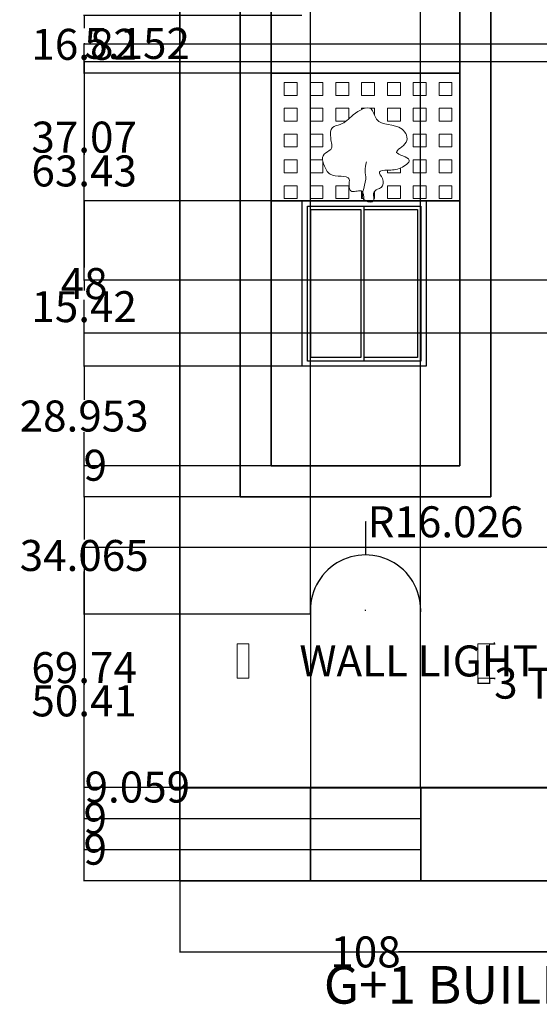
# Model space of a CAD drawing. Units: inches. Extents: x -30 to 323, y -174 to 256.
# Tile 1 of 4: x -24 to 127, y -174 to 112. Entities that reach past the tile are written whole.
import ezdxf

# ---------------------------------------------------------------- set-up
doc = ezdxf.new("R2010")
doc.units = ezdxf.units.IN
doc.header["$MEASUREMENT"] = 0
for name, color, linetype, lineweight in [('A-ANNO-DIMS', 2, 'Continuous', 18), ('A-ANNO-TEXT', 7, 'Continuous', 25), ('A-DOOR', 4, 'Continuous', 25), ('A-ELEV', 7, 'Continuous', 35), ('A-ELEV-PATT', 8, 'Continuous', 13), ('A-FLOR-STRS', 7, 'Continuous', 25), ('A-GLAZ', 3, 'Continuous', 25), ('E-LITE', 6, 'Continuous', 18), ('L-PLNT', 3, 'Continuous', 18)]:
    doc.layers.add(name, color=color, linetype=linetype, lineweight=lineweight)
doc.styles.get("Standard").update_dxf_attribs({"font": 'arial.ttf'})
doc.dimstyles.get("Standard").update_dxf_attribs({"dimtxt": 9, "dimasz": 0.18, "dimexe": 0.18, "dimexo": 0.0625, "dimgap": 0.09, "dimtad": 0, "dimtih": 1, "dimtoh": 1, "dimdec": 0, "dimzin": 0, "dimdsep": 46, "dimlunit": 3, "dimtxsty": 'Standard', "dimcen": 0.09, "dimadec": 0, "dimazin": 0, "dimtfac": 1, "dimtdec": 0, "dimtofl": 0, "dimtmove": 0, "dimatfit": 3, "dimfxl": 1, "dimtolj": 1, "dimtzin": 0, "dimarcsym": 0})

# ---------------------------------------------------------------- blocks, each defined once
blk = doc.blocks.new('*U2')
for p, q in [((1.5, 1.5), (1.5, 46.5)), ((1.5, 46.5), (18, 46.5)), ((18, 1.5), (18, 46.5)), ((18, 46.5), (34.5, 46.5)), ((34.5, 46.5), (34.5, 1.5)), ((18, 1.5), (1.5, 1.5)), ((34.5, 1.5), (18, 1.5))]:
    blk.add_line(p, q)
blk.add_lwpolyline([(0, 0), (0, 48), (36, 48), (36, 0)], close=True)
for points in [[(17, 45.5), (17, 2.5), (2.5, 2.5), (2.5, 45.5), (17, 45.5)], [(18, 45.5), (33.5, 45.5), (33.5, 2.5), (18, 2.5)]]:
    blk.add_lwpolyline(points)
blk = doc.blocks.new('WALL-LIGHT')
blk.add_lwpolyline([(0, 9.92), (3.36, 9.92), (3.36, 0), (0, 0)], close=True)
blk = doc.blocks.new('*D7')
at = {"layer": 'A-ANNO-DIMS', "color": 0, "lineweight": -2, "transparency": 16777216}
for p, q in [((112.24, -69.33), (113.85, -69.33)), ((113.67, -69.15), (113.67, -68.97)), ((112.24, -79.25), (113.85, -79.25)), ((113.67, -79.43), (113.67, -79.61))]:
    blk.add_line(p, q, dxfattribs=at)
at = {"layer": 'A-ANNO-DIMS', "color": 0, "transparency": 16777216}
for points in [[(113.64, -69.15), (113.7, -69.15), (113.67, -69.33)], [(113.64, -79.43), (113.7, -79.43), (113.67, -79.25)]]:
    blk.add_solid(points, dxfattribs=at)
at = {"layer": 'Defpoints', "color": 0, "transparency": 16777216}
for p in [(112.18, -69.33), (113.67, -69.33), (112.18, -79.25)]:
    blk.add_point(p, dxfattribs=at)
at = {"layer": 'A-ANNO-DIMS', "color": 0, "transparency": 16777216, "insert": (113.67, -74.29), "char_height": 9, "attachment_point": 5}
blk.add_mtext('\\A1;WALL LIGHT 10 TYP.', dxfattribs=at)
blk = doc.blocks.new('*D8')
at = {"layer": 'A-ANNO-DIMS', "color": 0, "lineweight": -2, "transparency": 16777216}
for p, q in [((108.82, -79.31), (108.82, -80.91)), ((112.18, -79.31), (112.18, -80.91)), ((109, -80.73), (112, -80.73)), ((112.18, -80.73), (112.36, -80.73))]:
    blk.add_line(p, q, dxfattribs=at)
at = {"layer": 'A-ANNO-DIMS', "color": 0, "transparency": 16777216}
for points in [[(109, -80.7), (109, -80.76), (108.82, -80.73)], [(112, -80.7), (112, -80.76), (112.18, -80.73)]]:
    blk.add_solid(points, dxfattribs=at)
at = {"layer": 'Defpoints', "color": 0, "transparency": 16777216}
for p in [(108.82, -79.25), (112.18, -79.25), (112.18, -80.73)]:
    blk.add_point(p, dxfattribs=at)
at = {"layer": 'A-ANNO-DIMS', "color": 0, "transparency": 16777216, "insert": (130.85, -80.73), "char_height": 9, "attachment_point": 5}
blk.add_mtext('\\A1;3 TYP.', dxfattribs=at)
blk = doc.blocks.new('*D9')
at = {"layer": 'A-ANNO-DIMS', "color": 0, "lineweight": -2, "transparency": 16777216}
for p, q in [((283.63, 8.84), (283.63, -158.98)), ((22.14, -138.22), (22.14, -158.98)), ((22.32, -158.8), (137.5, -158.8)), ((283.45, -158.8), (168.27, -158.8))]:
    blk.add_line(p, q, dxfattribs=at)
at = {"layer": 'A-ANNO-DIMS', "color": 0, "transparency": 16777216}
for points in [[(22.32, -158.77), (22.32, -158.83), (22.14, -158.8)], [(283.45, -158.77), (283.45, -158.83), (283.63, -158.8)]]:
    blk.add_solid(points, dxfattribs=at)
at = {"layer": 'Defpoints', "color": 0, "transparency": 16777216}
for p in [(283.63, 8.91), (22.14, -138.15), (283.63, -158.8)]:
    blk.add_point(p, dxfattribs=at)
at = {"layer": 'A-ANNO-DIMS', "color": 0, "transparency": 16777216, "insert": (152.88, -158.8), "char_height": 9, "attachment_point": 5}
blk.add_mtext('\\A1;261.5', dxfattribs=at)
blk = doc.blocks.new('*D10')
at = {"layer": 'A-ANNO-DIMS', "color": 0, "lineweight": -2, "transparency": 16777216}
for p, q in [((15.03, 229.9), (304.46, 229.9)), ((304.28, 229.72), (304.28, 50.56)), ((304.28, -137.97), (304.28, 41.18)), ((22.2, -138.15), (304.46, -138.15))]:
    blk.add_line(p, q, dxfattribs=at)
at = {"layer": 'A-ANNO-DIMS', "color": 0, "transparency": 16777216}
for points in [[(304.25, 229.72), (304.31, 229.72), (304.28, 229.9)], [(304.25, -137.97), (304.31, -137.97), (304.28, -138.15)]]:
    blk.add_solid(points, dxfattribs=at)
at = {"layer": 'Defpoints', "color": 0, "transparency": 16777216}
for p in [(14.97, 229.9), (22.14, -138.15), (304.28, -138.15)]:
    blk.add_point(p, dxfattribs=at)
at = {"layer": 'A-ANNO-DIMS', "color": 0, "transparency": 16777216, "insert": (304.28, 45.87), "char_height": 9, "attachment_point": 5}
blk.add_mtext('\\A1;368.05', dxfattribs=at)
blk = doc.blocks.new('*D21')
at = {"layer": 'A-ANNO-DIMS', "color": 0, "lineweight": -2, "transparency": 16777216}
for p, q in [((22.14, -111.03), (22.14, 250.73)), ((22.32, 250.55), (25.92, 250.55)), ((59.97, 250.55), (56.37, 250.55)), ((60.15, -60.62), (60.15, 250.73))]:
    blk.add_line(p, q, dxfattribs=at)
at = {"layer": 'A-ANNO-DIMS', "color": 0, "transparency": 16777216}
for points in [[(22.32, 250.58), (22.32, 250.52), (22.14, 250.55)], [(59.97, 250.58), (59.97, 250.52), (60.15, 250.55)]]:
    blk.add_solid(points, dxfattribs=at)
at = {"layer": 'Defpoints', "color": 0, "transparency": 16777216}
for p in [(60.15, 250.55), (60.15, -60.68), (22.14, -111.09)]:
    blk.add_point(p, dxfattribs=at)
at = {"layer": 'A-ANNO-DIMS', "color": 0, "transparency": 16777216, "insert": (41.14, 250.55), "char_height": 9, "attachment_point": 5}
blk.add_mtext('\\A1;38.02', dxfattribs=at)
blk = doc.blocks.new('*D22')
at = {"layer": 'A-ANNO-DIMS', "color": 0, "lineweight": -2, "transparency": 16777216}
for p, q in [((92.12, -60.62), (92.12, 250.73)), ((92.3, 250.55), (95.9, 250.55)), ((129.96, 250.55), (126.35, 250.55)), ((130.14, -111.03), (130.14, 250.73))]:
    blk.add_line(p, q, dxfattribs=at)
at = {"layer": 'A-ANNO-DIMS', "color": 0, "transparency": 16777216}
for points in [[(92.3, 250.58), (92.3, 250.52), (92.12, 250.55)], [(129.96, 250.58), (129.96, 250.52), (130.14, 250.55)]]:
    blk.add_solid(points, dxfattribs=at)
at = {"layer": 'Defpoints', "color": 0, "transparency": 16777216}
for p in [(130.14, 250.55), (92.12, -60.68), (130.14, -111.09)]:
    blk.add_point(p, dxfattribs=at)
at = {"layer": 'A-ANNO-DIMS', "color": 0, "transparency": 16777216, "insert": (111.13, 250.55), "char_height": 9, "attachment_point": 5}
blk.add_mtext('\\A1;38.02', dxfattribs=at)
blk = doc.blocks.new('*D23')
at = {"layer": 'A-ANNO-DIMS', "color": 0, "lineweight": -2, "transparency": 16777216}
for p, q in [((22.14, -138.22), (22.14, -158.98)), ((130.14, -138.22), (130.14, -158.98)), ((22.32, -158.8), (66.52, -158.8)), ((129.96, -158.8), (85.75, -158.8))]:
    blk.add_line(p, q, dxfattribs=at)
at = {"layer": 'A-ANNO-DIMS', "color": 0, "transparency": 16777216}
for points in [[(22.32, -158.77), (22.32, -158.83), (22.14, -158.8)], [(129.96, -158.77), (129.96, -158.83), (130.14, -158.8)]]:
    blk.add_solid(points, dxfattribs=at)
at = {"layer": 'Defpoints', "color": 0, "transparency": 16777216}
for p in [(22.14, -138.15), (130.14, -138.15), (130.14, -158.8)]:
    blk.add_point(p, dxfattribs=at)
at = {"layer": 'A-ANNO-DIMS', "color": 0, "transparency": 16777216, "insert": (76.14, -158.8), "char_height": 9, "attachment_point": 5}
blk.add_mtext('\\A1;108', dxfattribs=at)
blk = doc.blocks.new('*D24')
at = {"layer": 'A-ANNO-DIMS', "color": 0, "lineweight": -2, "transparency": 16777216}
for p, q in [((60.09, -129.15), (-5.86, -129.15)), ((-5.68, -129.15), (-5.68, -128.97)), ((-5.68, -128.97), (-5.5, -128.97)), ((-5.68, -137.97), (-5.68, -129.33)), ((22.07, -138.15), (-5.86, -138.15))]:
    blk.add_line(p, q, dxfattribs=at)
at = {"layer": 'A-ANNO-DIMS', "color": 0, "transparency": 16777216}
for points in [[(-5.71, -129.33), (-5.65, -129.33), (-5.68, -129.15)], [(-5.71, -137.97), (-5.65, -137.97), (-5.68, -138.15)]]:
    blk.add_solid(points, dxfattribs=at)
at = {"layer": 'Defpoints', "color": 0, "transparency": 16777216}
for p in [(-5.68, -129.15), (60.15, -129.15), (22.14, -138.15)]:
    blk.add_point(p, dxfattribs=at)
at = {"layer": 'A-ANNO-DIMS', "color": 0, "transparency": 16777216, "insert": (-2.45, -128.97), "char_height": 9, "attachment_point": 5}
blk.add_mtext('\\A1;9', dxfattribs=at)
blk = doc.blocks.new('*D25')
at = {"layer": 'A-ANNO-DIMS', "color": 0, "lineweight": -2, "transparency": 16777216}
for p, q in [((-5.68, -120.15), (-5.68, -119.97)), ((-5.68, -119.97), (-5.5, -119.97)), ((60.09, -120.15), (-5.86, -120.15)), ((-5.68, -128.97), (-5.68, -120.33)), ((60.09, -129.15), (-5.86, -129.15))]:
    blk.add_line(p, q, dxfattribs=at)
at = {"layer": 'A-ANNO-DIMS', "color": 0, "transparency": 16777216}
for points in [[(-5.71, -120.33), (-5.65, -120.33), (-5.68, -120.15)], [(-5.71, -128.97), (-5.65, -128.97), (-5.68, -129.15)]]:
    blk.add_solid(points, dxfattribs=at)
at = {"layer": 'Defpoints', "color": 0, "transparency": 16777216}
for p in [(-5.68, -120.15), (60.15, -120.15), (60.15, -129.15)]:
    blk.add_point(p, dxfattribs=at)
at = {"layer": 'A-ANNO-DIMS', "color": 0, "transparency": 16777216, "insert": (-2.45, -119.97), "char_height": 9, "attachment_point": 5}
blk.add_mtext('\\A1;9', dxfattribs=at)
blk = doc.blocks.new('*D26')
at = {"layer": 'A-ANNO-DIMS', "color": 0, "lineweight": -2, "transparency": 16777216}
for p, q in [((22.07, -111.09), (-5.86, -111.09)), ((-5.68, -111.09), (-5.68, -110.91)), ((-5.68, -110.91), (-5.5, -110.91)), ((-5.68, -119.97), (-5.68, -111.27)), ((60.09, -120.15), (-5.86, -120.15))]:
    blk.add_line(p, q, dxfattribs=at)
at = {"layer": 'A-ANNO-DIMS', "color": 0, "transparency": 16777216}
for points in [[(-5.71, -111.27), (-5.65, -111.27), (-5.68, -111.09)], [(-5.71, -119.97), (-5.65, -119.97), (-5.68, -120.15)]]:
    blk.add_solid(points, dxfattribs=at)
at = {"layer": 'Defpoints', "color": 0, "transparency": 16777216}
for p in [(-5.68, -111.09), (22.14, -111.09), (60.15, -120.15)]:
    blk.add_point(p, dxfattribs=at)
at = {"layer": 'A-ANNO-DIMS', "color": 0, "transparency": 16777216, "insert": (9.78, -110.91), "char_height": 9, "attachment_point": 5}
blk.add_mtext('\\A1;9.059', dxfattribs=at)
blk = doc.blocks.new('*D27')
at = {"layer": 'A-ANNO-DIMS', "color": 0, "lineweight": -2, "transparency": 16777216}
for p, q in [((60.09, -60.68), (-5.86, -60.68)), ((-5.68, -60.86), (-5.68, -81.2)), ((-5.68, -110.91), (-5.68, -90.57)), ((22.07, -111.09), (-5.86, -111.09))]:
    blk.add_line(p, q, dxfattribs=at)
at = {"layer": 'A-ANNO-DIMS', "color": 0, "transparency": 16777216}
for points in [[(-5.71, -60.86), (-5.65, -60.86), (-5.68, -60.68)], [(-5.71, -110.91), (-5.65, -110.91), (-5.68, -111.09)]]:
    blk.add_solid(points, dxfattribs=at)
at = {"layer": 'Defpoints', "color": 0, "transparency": 16777216}
for p in [(-5.68, -60.68), (60.15, -60.68), (22.14, -111.09)]:
    blk.add_point(p, dxfattribs=at)
at = {"layer": 'A-ANNO-DIMS', "color": 0, "transparency": 16777216, "insert": (-5.68, -85.89), "char_height": 9, "attachment_point": 5}
blk.add_mtext('\\A1;50.41', dxfattribs=at)
blk = doc.blocks.new('*D28')
at = {"layer": 'A-ANNO-DIMS', "color": 0, "lineweight": -2, "transparency": 16777216}
for p, q in [((39.63, -26.62), (-5.86, -26.62)), ((-5.68, -26.8), (-5.68, -38.96)), ((-5.68, -60.5), (-5.68, -48.34)), ((60.09, -60.68), (-5.86, -60.68))]:
    blk.add_line(p, q, dxfattribs=at)
at = {"layer": 'A-ANNO-DIMS', "color": 0, "transparency": 16777216}
for points in [[(-5.71, -26.8), (-5.65, -26.8), (-5.68, -26.62)], [(-5.71, -60.5), (-5.65, -60.5), (-5.68, -60.68)]]:
    blk.add_solid(points, dxfattribs=at)
at = {"layer": 'Defpoints', "color": 0, "transparency": 16777216}
for p in [(-5.68, -26.62), (39.69, -26.62), (60.15, -60.68)]:
    blk.add_point(p, dxfattribs=at)
at = {"layer": 'A-ANNO-DIMS', "color": 0, "transparency": 16777216, "insert": (-5.68, -43.65), "char_height": 9, "attachment_point": 5}
blk.add_mtext('\\A1;34.065', dxfattribs=at)
blk = doc.blocks.new('*D29')
at = {"layer": 'A-ANNO-DIMS', "color": 0, "lineweight": -2, "transparency": 16777216}
for p, q in [((48.63, -17.62), (-5.86, -17.62)), ((-5.68, -17.62), (-5.68, -17.44)), ((-5.68, -17.44), (-5.5, -17.44)), ((-5.68, -26.44), (-5.68, -17.8)), ((39.63, -26.62), (-5.86, -26.62))]:
    blk.add_line(p, q, dxfattribs=at)
at = {"layer": 'A-ANNO-DIMS', "color": 0, "transparency": 16777216}
for points in [[(-5.71, -17.8), (-5.65, -17.8), (-5.68, -17.62)], [(-5.71, -26.44), (-5.65, -26.44), (-5.68, -26.62)]]:
    blk.add_solid(points, dxfattribs=at)
at = {"layer": 'Defpoints', "color": 0, "transparency": 16777216}
for p in [(-5.68, -17.62), (48.69, -17.62), (39.69, -26.62)]:
    blk.add_point(p, dxfattribs=at)
at = {"layer": 'A-ANNO-DIMS', "color": 0, "transparency": 16777216, "insert": (-2.45, -17.44), "char_height": 9, "attachment_point": 5}
blk.add_mtext('\\A1;9', dxfattribs=at)
blk = doc.blocks.new('*D30')
at = {"layer": 'A-ANNO-DIMS', "color": 0, "lineweight": -2, "transparency": 16777216}
for p, q in [((57.66, 11.33), (-5.86, 11.33)), ((-5.68, 11.15), (-5.68, 1.55)), ((-5.68, -17.44), (-5.68, -7.83)), ((48.63, -17.62), (-5.86, -17.62))]:
    blk.add_line(p, q, dxfattribs=at)
at = {"layer": 'A-ANNO-DIMS', "color": 0, "transparency": 16777216}
for points in [[(-5.71, 11.15), (-5.65, 11.15), (-5.68, 11.33)], [(-5.71, -17.44), (-5.65, -17.44), (-5.68, -17.62)]]:
    blk.add_solid(points, dxfattribs=at)
at = {"layer": 'Defpoints', "color": 0, "transparency": 16777216}
for p in [(-5.68, 11.33), (57.72, 11.33), (48.69, -17.62)]:
    blk.add_point(p, dxfattribs=at)
at = {"layer": 'A-ANNO-DIMS', "color": 0, "transparency": 16777216, "insert": (-5.68, -3.14), "char_height": 9, "attachment_point": 5}
blk.add_mtext('\\A1;28.953', dxfattribs=at)
blk = doc.blocks.new('*D31')
at = {"layer": 'A-ANNO-DIMS', "color": 0, "lineweight": -2, "transparency": 16777216}
for p, q in [((48.63, 59.33), (-5.86, 59.33)), ((-5.68, 59.15), (-5.68, 40.02)), ((-5.68, 11.51), (-5.68, 30.65)), ((57.66, 11.33), (-5.86, 11.33))]:
    blk.add_line(p, q, dxfattribs=at)
at = {"layer": 'A-ANNO-DIMS', "color": 0, "transparency": 16777216}
for points in [[(-5.71, 59.15), (-5.65, 59.15), (-5.68, 59.33)], [(-5.71, 11.51), (-5.65, 11.51), (-5.68, 11.33)]]:
    blk.add_solid(points, dxfattribs=at)
at = {"layer": 'Defpoints', "color": 0, "transparency": 16777216}
for p in [(-5.68, 59.33), (48.7, 59.33), (57.72, 11.33)]:
    blk.add_point(p, dxfattribs=at)
at = {"layer": 'A-ANNO-DIMS', "color": 0, "transparency": 16777216, "insert": (-5.68, 35.33), "char_height": 9, "attachment_point": 5}
blk.add_mtext('\\A1;48', dxfattribs=at)
blk = doc.blocks.new('*D32')
at = {"layer": 'A-ANNO-DIMS', "color": 0, "lineweight": -2, "transparency": 16777216}
for p, q in [((48.63, 96.41), (-5.86, 96.41)), ((-5.68, 96.23), (-5.68, 82.56)), ((-5.68, 59.51), (-5.68, 73.18)), ((48.63, 59.33), (-5.86, 59.33))]:
    blk.add_line(p, q, dxfattribs=at)
at = {"layer": 'A-ANNO-DIMS', "color": 0, "transparency": 16777216}
for points in [[(-5.71, 96.23), (-5.65, 96.23), (-5.68, 96.41)], [(-5.71, 59.51), (-5.65, 59.51), (-5.68, 59.33)]]:
    blk.add_solid(points, dxfattribs=at)
at = {"layer": 'Defpoints', "color": 0, "transparency": 16777216}
for p in [(-5.68, 96.41), (48.7, 96.41), (48.7, 59.33)]:
    blk.add_point(p, dxfattribs=at)
at = {"layer": 'A-ANNO-DIMS', "color": 0, "transparency": 16777216, "insert": (-5.68, 77.87), "char_height": 9, "attachment_point": 5}
blk.add_mtext('\\A1;37.07', dxfattribs=at)
blk = doc.blocks.new('*D33')
at = {"layer": 'A-ANNO-DIMS', "color": 0, "lineweight": -2, "transparency": 16777216}
for p, q in [((57.66, 113.23), (-5.86, 113.23)), ((-5.68, 113.05), (-5.68, 109.5)), ((-5.68, 96.59), (-5.68, 100.13)), ((48.63, 96.41), (-5.86, 96.41))]:
    blk.add_line(p, q, dxfattribs=at)
at = {"layer": 'A-ANNO-DIMS', "color": 0, "transparency": 16777216}
for points in [[(-5.71, 113.05), (-5.65, 113.05), (-5.68, 113.23)], [(-5.71, 96.59), (-5.65, 96.59), (-5.68, 96.41)]]:
    blk.add_solid(points, dxfattribs=at)
at = {"layer": 'Defpoints', "color": 0, "transparency": 16777216}
for p in [(-5.68, 113.23), (57.72, 113.23), (48.7, 96.41)]:
    blk.add_point(p, dxfattribs=at)
at = {"layer": 'A-ANNO-DIMS', "color": 0, "transparency": 16777216, "insert": (-5.68, 104.82), "char_height": 9, "attachment_point": 5}
blk.add_mtext('\\A1;16.82', dxfattribs=at)
blk = doc.blocks.new('*D61')
at = {"layer": 'A-ANNO-DIMS', "color": 0, "lineweight": -2, "transparency": 16777216}
for p, q in [((148.07, -41.35), (-5.86, -41.35)), ((-5.68, -41.53), (-5.68, -71.54)), ((-5.68, -110.91), (-5.68, -80.91)), ((130.07, -111.09), (-5.86, -111.09))]:
    blk.add_line(p, q, dxfattribs=at)
at = {"layer": 'A-ANNO-DIMS', "color": 0, "transparency": 16777216}
for points in [[(-5.71, -41.53), (-5.65, -41.53), (-5.68, -41.35)], [(-5.71, -110.91), (-5.65, -110.91), (-5.68, -111.09)]]:
    blk.add_solid(points, dxfattribs=at)
at = {"layer": 'Defpoints', "color": 0, "transparency": 16777216}
for p in [(-5.68, -41.35), (148.14, -41.35), (130.14, -111.09)]:
    blk.add_point(p, dxfattribs=at)
at = {"layer": 'A-ANNO-DIMS', "color": 0, "transparency": 16777216, "insert": (-5.68, -76.22), "char_height": 9, "attachment_point": 5}
blk.add_mtext('\\A1;69.74', dxfattribs=at)
blk = doc.blocks.new('*D74')
at = {"layer": 'A-ANNO-DIMS', "color": 0, "lineweight": -2, "transparency": 16777216}
for p, q in [((145.92, 36.33), (-5.86, 36.33)), ((-5.68, 36.15), (-5.68, 33.3)), ((-5.68, 21.09), (-5.68, 23.93)), ((142.07, 20.91), (-5.86, 20.91))]:
    blk.add_line(p, q, dxfattribs=at)
at = {"layer": 'A-ANNO-DIMS', "color": 0, "transparency": 16777216}
for points in [[(-5.71, 36.15), (-5.65, 36.15), (-5.68, 36.33)], [(-5.71, 21.09), (-5.65, 21.09), (-5.68, 20.91)]]:
    blk.add_solid(points, dxfattribs=at)
at = {"layer": 'Defpoints', "color": 0, "transparency": 16777216}
for p in [(-5.68, 36.33), (145.99, 36.33), (142.14, 20.91)]:
    blk.add_point(p, dxfattribs=at)
at = {"layer": 'A-ANNO-DIMS', "color": 0, "transparency": 16777216, "insert": (-5.68, 28.62), "char_height": 9, "attachment_point": 5}
blk.add_mtext('\\A1;15.42', dxfattribs=at)
blk = doc.blocks.new('*D75')
at = {"layer": 'A-ANNO-DIMS', "color": 0, "lineweight": -2, "transparency": 16777216}
for p, q in [((145.92, 99.75), (-5.86, 99.75)), ((-5.68, 99.57), (-5.68, 72.73)), ((-5.68, 36.51), (-5.68, 63.35)), ((145.92, 36.33), (-5.86, 36.33))]:
    blk.add_line(p, q, dxfattribs=at)
at = {"layer": 'A-ANNO-DIMS', "color": 0, "transparency": 16777216}
for points in [[(-5.71, 99.57), (-5.65, 99.57), (-5.68, 99.75)], [(-5.71, 36.51), (-5.65, 36.51), (-5.68, 36.33)]]:
    blk.add_solid(points, dxfattribs=at)
at = {"layer": 'Defpoints', "color": 0, "transparency": 16777216}
for p in [(-5.68, 99.75), (145.99, 99.75), (145.99, 36.33)]:
    blk.add_point(p, dxfattribs=at)
at = {"layer": 'A-ANNO-DIMS', "color": 0, "transparency": 16777216, "insert": (-5.68, 68.04), "char_height": 9, "attachment_point": 5}
blk.add_mtext('\\A1;63.43', dxfattribs=at)
blk = doc.blocks.new('*D76')
at = {"layer": 'A-ANNO-DIMS', "color": 0, "lineweight": -2, "transparency": 16777216}
for p, q in [((142.07, 104.91), (-5.86, 104.91)), ((-5.68, 104.91), (-5.68, 105.09)), ((-5.68, 105.09), (-5.5, 105.09)), ((-5.68, 99.93), (-5.68, 104.73)), ((145.92, 99.75), (-5.86, 99.75))]:
    blk.add_line(p, q, dxfattribs=at)
at = {"layer": 'A-ANNO-DIMS', "color": 0, "transparency": 16777216}
for points in [[(-5.71, 104.73), (-5.65, 104.73), (-5.68, 104.91)], [(-5.71, 99.93), (-5.65, 99.93), (-5.68, 99.75)]]:
    blk.add_solid(points, dxfattribs=at)
at = {"layer": 'Defpoints', "color": 0, "transparency": 16777216}
for p in [(-5.68, 104.91), (142.14, 104.91), (145.99, 99.75)]:
    blk.add_point(p, dxfattribs=at)
at = {"layer": 'A-ANNO-DIMS', "color": 0, "transparency": 16777216, "insert": (9.73, 105.09), "char_height": 9, "attachment_point": 5}
blk.add_mtext('\\A1;5.152', dxfattribs=at)
blk = doc.blocks.new('*D77')
at = {"layer": 'A-ANNO-DIMS', "color": 0, "lineweight": -2, "transparency": 16777216}
for p, q in [((76.32, -33.87), (76.14, -33.87)), ((76.14, -33.87), (76.14, -43.3)), ((76.05, -59.51), (76.23, -59.51)), ((76.14, -59.6), (76.14, -59.42))]:
    blk.add_line(p, q, dxfattribs=at)
at = {"layer": 'A-ANNO-DIMS', "color": 0, "transparency": 16777216}
blk.add_solid([(76.11, -43.3), (76.17, -43.3), (76.14, -43.48)], dxfattribs=at)
at = {"layer": 'Defpoints', "color": 0, "transparency": 16777216}
for p in [(76.14, -43.48), (76.14, -59.51)]:
    blk.add_point(p, dxfattribs=at)
at = {"layer": 'A-ANNO-DIMS', "color": 0, "transparency": 16777216, "insert": (99.39, -33.87), "char_height": 9, "attachment_point": 5}
blk.add_mtext('\\A1;R16.026', dxfattribs=at)

msp = doc.modelspace()

# ---------------------------------------------------------------- hatches: boundary and pattern name
at = {"layer": 'A-ELEV-PATT'}
h = msp.add_hatch(dxfattribs=at)
h.set_pattern_fill('SQUARE', color=256, scale=30)
edge = h.paths.add_edge_path()
edge.add_spline(control_points=[(75.3211, 61.7995), (75.1986, 62.0071), (74.4578, 62.6896), (71.738, 61.3333), (71.2119, 63.9023), (72.0257, 67.3627), (66.4586, 65.797), (64.2082, 69.0428), (62.6837, 72.8814), (66.9111, 74.1759), (65.8088, 77.508), (65.831, 81.0228), (69.831, 81.5148), (72.1684, 84.4623), (78.0553, 87.8418), (79.2681, 80.5196), (86.2826, 82.5145), (89.4686, 76.0117), (82.5196, 73.1865), (90.9262, 71.7358), (85.7413, 68.2966), (83.5112, 68.3268), (79.2817, 68.145), (81.5493, 65.7412), (81.2688, 63.2947), (79.4617, 62.7519), (77.8918, 61.5997), (78.7703, 59.7999), (78.4437, 59.334)], knot_values=[2.20389569, 2.20389569, 2.20389569, 2.20389569, 3.0333133, 5.96980343, 7.60712091, 9.50541194, 15.20272299, 16.79439629, 21.50478909, 23.85346698, 27.13233668, 30.28156068, 32.68718212, 37.38454327, 42.8463849, 46.16655969, 54.15254193, 58.13701982, 62.16754012, 66.43266235, 69.73131729, 73.76374154, 76.06819784, 78.15373141, 80.76526319, 81.92378142, 83.63296344, 85.8374237, 85.8374237, 85.8374237, 85.8374237], degree=3, periodic=0)
edge.add_line((78.4437, 59.334), (93.7226, 59.334))
edge.add_line((93.7226, 59.334), (103.581, 59.334))
edge.add_line((103.581, 59.334), (103.5822, 96.4058))
edge.add_line((103.5822, 96.4058), (48.6979, 96.4058))
edge.add_line((48.6979, 96.4058), (48.6966, 59.334))
edge.add_line((48.6966, 59.334), (75.7226, 59.334))
edge.add_spline(control_points=[(75.7226, 59.334), (75.7185, 59.4366), (75.7144, 59.5392), (75.71, 59.6412)], knot_values=[0, 0, 0, 0, 0.23624815, 0.23624815, 0.23624815, 0.23624815], degree=3, periodic=0)
edge.add_spline(control_points=[(75.71, 59.6412), (75.1902, 60.1562), (75.1644, 60.926), (75.3211, 61.7995)], knot_values=[88.68438083, 88.68438083, 88.68438083, 88.68438083, 91.0965344, 91.0965344, 91.0965344, 91.0965344], degree=3, periodic=0)

# ---------------------------------------------------------------- linework, layer by layer
at = {"layer": 'A-DOOR'}
msp.add_lwpolyline([(60.1531, -60.6838), (60.1531, -111.0941), (92.1189, -111.0941), (92.1189, -60.6838, 1.07623618)], format="xyb", close=True, dxfattribs=at)
at = {"layer": 'A-ELEV'}
for p, q in [((39.6938, -26.6189), (39.7012, 195.2341)), ((112.5855, 195.2341), (112.5782, -26.6189)), ((48.6941, -17.6189), (48.7009, 186.2341)), ((103.5852, 186.2341), (103.5785, -17.6189)), ((103.5785, -17.6189), (48.6941, -17.6189)), ((112.5782, -26.6189), (39.6938, -26.6189))]:
    msp.add_line(p, q, dxfattribs=at)
msp.add_lwpolyline([(130.136, 149.9059), (274.136, 149.9059), (274.136, 128.9059), (279.5695, 128.9059), (279.5695, 104.9059), (274.136, 104.9059), (274.136, 20.9059), (283.6325, 20.9059), (283.6325, 8.9059), (274.136, 8.9059), (274.136, -111.0941), (22.136, -111.0941), (22.136, 224.9059), (130.136, 224.9059), (130.136, -111.0941)], dxfattribs=at)
for points in [[(48.6966, 59.334), (103.5822, 59.334), (103.5822, 96.4058), (48.6966, 96.4058)], [(60.1531, -111.0941), (22.136, -111.0941), (22.136, -138.1526), (60.1531, -138.1526)], [(92.2427, -111.0941), (130.136, -111.0941), (130.136, -138.1526), (92.2427, -138.1526)]]:
    msp.add_lwpolyline(points, close=True, dxfattribs=at)
at = {"layer": 'A-FLOR-STRS'}
for p, q in [((60.1531, -138.1526), (60.1531, -111.0941)), ((92.2427, -111.0941), (92.2427, -138.1526)), ((92.2427, -120.1526), (60.1531, -120.1526)), ((92.2427, -129.1526), (60.1531, -129.1526)), ((92.2427, -138.1526), (60.1531, -138.1526))]:
    msp.add_line(p, q, dxfattribs=at)
at = {"layer": 'L-PLNT'}
msp.add_open_spline([(75.7226, 59.334), (75.6702, 60.651), (75.5671, 63.2427), (71.738, 61.3333), (71.2119, 63.9023), (72.0257, 67.3627), (66.4586, 65.797), (64.2082, 69.0428), (62.6837, 72.8814), (66.9111, 74.1759), (65.8088, 77.508), (65.831, 81.0228), (69.831, 81.5148), (72.1684, 84.4623), (78.0553, 87.8418), (79.2681, 80.5196), (86.2826, 82.5145), (89.4686, 76.0117), (82.5196, 73.1865), (90.9262, 71.7358), (85.7413, 68.2966), (83.5112, 68.3268), (79.2817, 68.145), (81.5493, 65.7412), (81.2688, 63.2947), (79.4617, 62.7519), (77.8918, 61.5997), (79.2875, 58.7402), (73.4514, 59.2667), (76.786, 64.556), (75.8288, 68.1331), (76.1857, 69.8132), (76.3709, 70.6848)], degree=3, knots=[0, 0, 0, 0, 3.0333133, 5.96980343, 7.60712091, 9.50541194, 15.20272299, 16.79439629, 21.50478909, 23.85346698, 27.13233668, 30.28156068, 32.68718212, 37.38454327, 42.8463849, 46.16655969, 54.15254193, 58.13701982, 62.16754012, 66.43266235, 69.73131729, 73.76374154, 76.06819784, 78.15373141, 80.76526319, 81.92378142, 83.63296344, 85.8374237, 88.14168399, 94.48814382, 96.91031937, 99.52185115, 99.52185115, 99.52185115, 99.52185115], dxfattribs=at)

# ---------------------------------------------------------------- block references
at = {"layer": 'A-GLAZ'}
msp.add_blockref('*U2', (57.7226, 11.334), dxfattribs=at)
at = {"layer": 'E-LITE'}
for p in [(38.841, -79.246), (108.8156, -79.246)]:
    msp.add_blockref('WALL-LIGHT', p, dxfattribs=at)

# ---------------------------------------------------------------- texts
at = {"layer": 'A-ANNO-TEXT'}
msp.add_text('G+1 BUILDING ELEVATION', height=10.938735, dxfattribs=at).set_placement((64.0004, -173.8227))

# ---------------------------------------------------------------- dimensions: what is measured, and where the dimension line sits
at = {"layer": 'A-ANNO-DIMS'}
for base, p1, p2, override, picture, middle in [((60.1531, 250.5457), (22.136, -111.0941), (60.1531, -60.6838), {"dimdec": 2, "dimlfac": 1, "dimrnd": 0, "dimzin": 0, "dimdsep": 46, "dimlunit": 2}, '*D21', (41.1445, 250.5457)), ((130.136, 250.5457), (92.1189, -60.6838), (130.136, -111.0941), {"dimdec": 2, "dimlfac": 1, "dimrnd": 0, "dimzin": 0, "dimdsep": 46, "dimlunit": 2}, '*D22', (111.1274, 250.5457)), ((283.6325, -158.8026), (22.136, -138.1526), (283.6325, 8.9059), {"dimdec": 1, "dimlfac": 1, "dimrnd": 0, "dimzin": 0, "dimdsep": 46, "dimlunit": 2}, '*D9', (152.8843, -158.8026)), ((130.136, -158.8026), (22.136, -138.1526), (130.136, -138.1526), {"dimdec": 0, "dimlfac": 1, "dimrnd": 0, "dimzin": 0, "dimdsep": 46, "dimlunit": 2}, '*D23', (76.136, -158.8026))]:
    dim = msp.add_linear_dim(base=base, p1=p1, p2=p2, dimstyle='Standard', override=override, dxfattribs=at)
    dim.commit()
    dim.dimension.update_dxf_attribs({"geometry": picture, "text_midpoint": middle})
for base, p1, p2, override, picture, middle in [((304.2825, -138.1526), (14.9689, 229.8957), (22.136, -138.1526), {"dimdec": 2, "dimlfac": 1, "dimrnd": 0, "dimzin": 0, "dimdsep": 46, "dimlunit": 2}, '*D10', (304.2825, 45.8715)), ((-5.6811, 113.2271), (48.6966, 96.4058), (57.7226, 113.2271), {"dimdec": 2, "dimlfac": 1, "dimrnd": 0, "dimzin": 0, "dimdsep": 46, "dimlunit": 2}, '*D33', (-5.6811, 104.8165)), ((-5.6811, 104.9059), (145.9862, 99.7543), (142.136, 104.9059), {"dimdec": 3, "dimlfac": 1, "dimrnd": 0, "dimzin": 0, "dimdsep": 46, "dimlunit": 2}, '*D76', (9.7281, 105.0859)), ((-5.6811, 99.7543), (145.9862, 36.3257), (145.9862, 99.7543), {"dimdec": 2, "dimlfac": 1, "dimrnd": 0, "dimzin": 0, "dimdsep": 46, "dimlunit": 2}, '*D75', (-5.6811, 68.04)), ((-5.6811, 96.4058), (48.6966, 59.334), (48.6966, 96.4058), {"dimdec": 2, "dimlfac": 1, "dimrnd": 0, "dimzin": 0, "dimdsep": 46, "dimlunit": 2}, '*D32', (-5.6811, 77.8699)), ((-5.6811, 59.334), (57.7226, 11.334), (48.6966, 59.334), {"dimdec": 0, "dimlfac": 1, "dimrnd": 0, "dimzin": 0, "dimdsep": 46, "dimlunit": 2}, '*D31', (-5.6811, 35.334)), ((-5.6811, 36.3257), (142.136, 20.9059), (145.9862, 36.3257), {"dimdec": 2, "dimlfac": 1, "dimrnd": 0, "dimzin": 0, "dimdsep": 46, "dimlunit": 2}, '*D74', (-5.6811, 28.6158)), ((-5.6811, 11.334), (48.6941, -17.6189), (57.7226, 11.334), {"dimdec": 3, "dimlfac": 1, "dimrnd": 0, "dimzin": 0, "dimdsep": 46, "dimlunit": 2}, '*D30', (-5.6811, -3.1424)), ((-5.6811, -17.6189), (39.6938, -26.6189), (48.6941, -17.6189), {"dimdec": 0, "dimlfac": 1, "dimrnd": 0, "dimzin": 0, "dimdsep": 46, "dimlunit": 2}, '*D29', (-2.452, -17.4389)), ((-5.6811, -26.6189), (60.1531, -60.6838), (39.6938, -26.6189), {"dimdec": 3, "dimlfac": 1, "dimrnd": 0, "dimzin": 0, "dimdsep": 46, "dimlunit": 2}, '*D28', (-5.6811, -43.6513)), ((-5.6811, -41.3495), (130.136, -111.0941), (148.136, -41.3495), {"dimdec": 2, "dimlfac": 1, "dimrnd": 0, "dimzin": 0, "dimdsep": 46, "dimlunit": 2}, '*D61', (-5.6811, -76.2218)), ((-5.6811, -60.6838), (22.136, -111.0941), (60.1531, -60.6838), {"dimdec": 2, "dimlfac": 1, "dimrnd": 0, "dimzin": 0, "dimdsep": 46, "dimlunit": 2}, '*D27', (-5.6811, -85.8889)), ((-5.68108, -111.09408), (60.15306, -120.15263), (22.13598, -111.09408), {"dimdec": 3, "dimlfac": 1, "dimrnd": 0, "dimzin": 0, "dimdsep": 46, "dimlunit": 2}, '*D26', (9.78333, -110.91408)), ((-5.6811, -120.1526), (60.1531, -129.1526), (60.1531, -120.1526), {"dimdec": 0, "dimlfac": 1, "dimrnd": 0, "dimzin": 0, "dimdsep": 46, "dimlunit": 2}, '*D25', (-2.452, -119.9726)), ((-5.6811, -129.1526), (22.136, -138.1526), (60.1531, -129.1526), {"dimdec": 0, "dimlfac": 1, "dimrnd": 0, "dimzin": 0, "dimdsep": 46, "dimlunit": 2}, '*D24', (-2.452, -128.9726))]:
    dim = msp.add_linear_dim(base=base, p1=p1, p2=p2, angle=90, dimstyle='Standard', override=override, dxfattribs=at)
    dim.commit()
    dim.dimension.update_dxf_attribs({"geometry": picture, "text_midpoint": middle})
dim = msp.add_radius_dim(center=(76.136, -59.5085), mpoint=(76.136, -43.4824), dimstyle='Standard', override={"dimdec": 3, "dimlfac": 1, "dimrnd": 0, "dimzin": 0, "dimdsep": 46, "dimlunit": 2}, dxfattribs=at)
dim.commit()
dim.dimension.update_dxf_attribs({"geometry": '*D77', "text_midpoint": (99.391, -33.8668), "dimtype": 164})
dim = msp.add_linear_dim(base=(113.6666, -69.3307), p1=(112.1793, -79.2457), p2=(112.1793, -69.3307), angle=90, text='WALL LIGHT <> TYP.', dimstyle='Standard', override={"dimdec": 0, "dimlfac": 1, "dimrnd": 0, "dimzin": 0, "dimdsep": 46, "dimlunit": 2}, dxfattribs=at)
dim.commit()
dim.dimension.update_dxf_attribs({"geometry": '*D7', "text_midpoint": (113.6666, -74.2882)})
dim = msp.add_linear_dim(base=(112.1793, -80.7329), p1=(108.8152, -79.2457), p2=(112.1793, -79.2457), text='<> TYP.', dimstyle='Standard', override={"dimdec": 0, "dimlfac": 1, "dimrnd": 0, "dimzin": 0, "dimdsep": 46, "dimlunit": 2}, dxfattribs=at)
dim.commit()
dim.dimension.update_dxf_attribs({"geometry": '*D8', "text_midpoint": (130.8545, -80.7329)})

doc.saveas('drawing.dxf')
